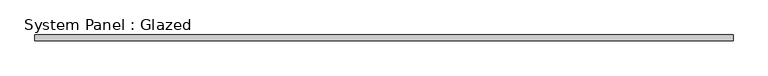
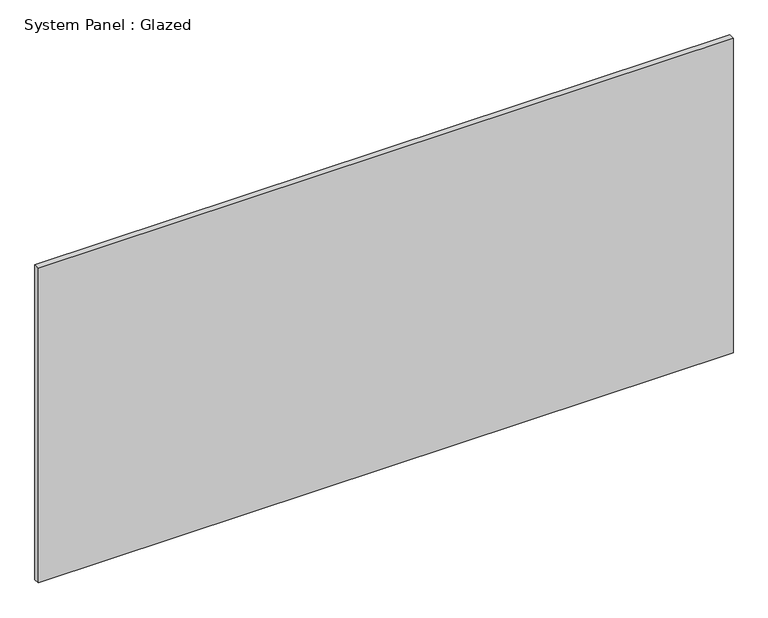
"""IFC4 building model written with IfcOpenShell, lengths in millimetres: plate geometry, System Panel : Glazed."""

from ifc_helpers import new_model, si_unit, origin, origin_with_axes, place, context, project, spatial, polyline, outline, extrude, source, transform, mapped, element, save


def system_panel_glazed_3620f98e(model_context):
    return source(origin(), model_context, "Body", "SweptSolid", [
        extrude(outline(polyline([(1492.25, 19.05), (-1492.25, 19.05), (-1492.25, 44.45), (1492.25, 44.45), (1492.25, 19.05)])), origin_with_axes(), (0.0, 0.0, 1.0), 1428.75),
    ])


if __name__ == "__main__":
    model = new_model("IFC4")
    model_context = context("Model", 3, world=origin())
    ifc_project = project(units=[si_unit("LENGTHUNIT", "METRE", prefix="MILLI")], contexts=[model_context])
    site = spatial("IfcSite", under=ifc_project)
    building = spatial("IfcBuilding", under=site)
    placement = place(None, origin())
    system_panel_glazed_shape = system_panel_glazed_3620f98e(model_context)
    element("IfcPlate", 1, ObjectType="System Panel : Glazed", at=placement, inside=building, context=model_context, shape_type="MappedRepresentation", body=[
        mapped(system_panel_glazed_shape, transform((0.0, 0.0, 0.0), x_axis=(1.0, 0.0, 0.0), y_axis=(0.0, 1.0, 0.0), z_axis=(0.0, 0.0, 1.0))),
    ])
    save(model, "model.ifc")

# Revit data of these elements
# Type "System Panel : Glazed"
#   Construction Type Id = "GSP4R"
#   Analytic Construction = "1/8 in Pilkington single glazing"
#   Visual Light Transmittance = 0.9
#   Solar Heat Gain Coefficient = 0.86
#   Heat Transfer Coefficient (U) = 1.18115 BTU/(h·ft²·°F)
#   Define Thermal Properties by = 1
# Element 1 (IfcPlate, "System Panel : Glazed")
#   Materials on its faces: "Glass"
# Materials
#   "Glass": class "Glass", colour RGB 0 128 192, transparency 0.75, Description = "Soda Lime Glass", Cost = 0
